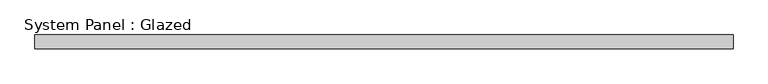
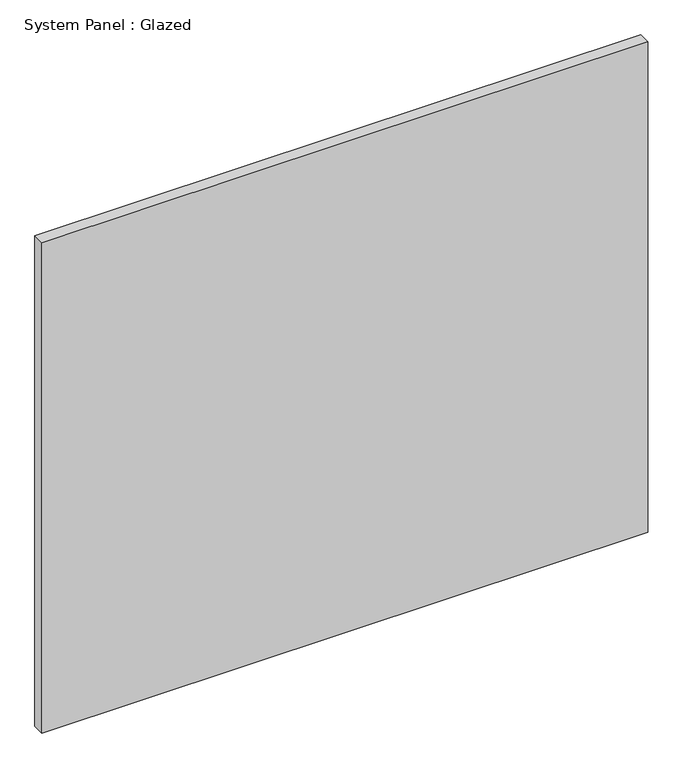
"""IFC4 building model written with IfcOpenShell, lengths in millimetres: plate geometry, System Panel : Glazed."""

from ifc_helpers import new_model, si_unit, origin, origin_with_axes, place, context, project, spatial, polyline, outline, extrude, source, transform, mapped, element, save


def system_panel_glazed_1b15d1ca(model_context):
    return source(origin(), model_context, "Body", "SweptSolid", [
        extrude(outline(polyline([(638.175, 19.05), (-638.175, 19.05), (-638.175, 44.45), (638.175, 44.45), (638.175, 19.05)])), origin_with_axes(), (0.0, 0.0, 1.0), 1092.2),
    ])


if __name__ == "__main__":
    model = new_model("IFC4")
    model_context = context("Model", 3, world=origin())
    ifc_project = project(units=[si_unit("LENGTHUNIT", "METRE", prefix="MILLI")], contexts=[model_context])
    site = spatial("IfcSite", under=ifc_project)
    building = spatial("IfcBuilding", under=site)
    placement = place(None, origin())
    system_panel_glazed_shape = system_panel_glazed_1b15d1ca(model_context)
    element("IfcPlate", 1, ObjectType="System Panel : Glazed", at=placement, inside=building, context=model_context, shape_type="MappedRepresentation", body=[
        mapped(system_panel_glazed_shape, transform((0.0, 0.0, 0.0), x_axis=(1.0, 0.0, 0.0), y_axis=(0.0, 1.0, 0.0), z_axis=(0.0, 0.0, 1.0))),
    ])
    save(model, "model.ifc")

# Revit data of these elements
# Type "System Panel : Glazed"
#   Construction Type Id = "GSP4R"
#   Analytic Construction = "1/8 in Pilkington single glazing"
#   Visual Light Transmittance = 0.9
#   Solar Heat Gain Coefficient = 0.86
#   Heat Transfer Coefficient (U) = 1.18115 BTU/(h·ft²·°F)
#   Define Thermal Properties by = 1
# Element 1 (IfcPlate, "System Panel : Glazed")
#   Materials on its faces: "Glass"
# Materials
#   "Glass": class "Glass", colour RGB 0 128 192, transparency 0.75, Description = "Soda Lime Glass", Cost = 0
